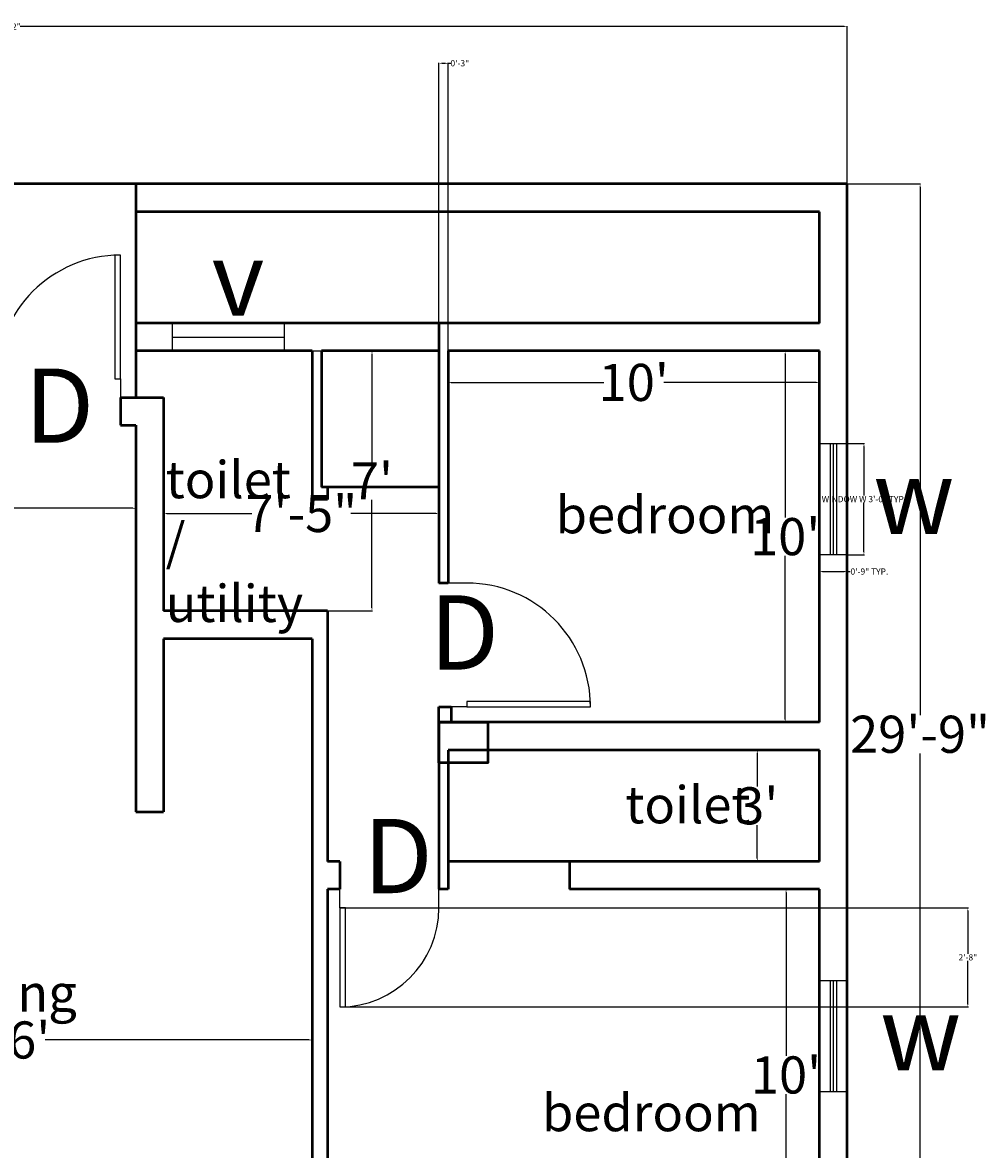
# Model space of a CAD drawing. Units: inches. Extents: x 409 to 7572, y 7 to 725.
# Tile 6 of 38: x 860 to 1171, y 360 to 725. Entities that reach past the tile are written whole.
import ezdxf

# ---------------------------------------------------------------- set-up
doc = ezdxf.new("R2010")
doc.units = ezdxf.units.IN
doc.header["$MEASUREMENT"] = 0
for name, color, linetype, lineweight in [('A-ANNO-DIMS', 2, 'Continuous', 18), ('A-ANNO-SYMB', 3, 'Continuous', 25), ('A-AREA-IDEN', 7, 'Continuous', 25), ('A-DOOR', 3, 'Continuous', 25), ('A-GLAZ', 4, 'Continuous', 25), ('A-WALL', 7, 'Continuous', 50)]:
    doc.layers.add(name, color=color, linetype=linetype, lineweight=lineweight)
doc.styles.get("Standard").update_dxf_attribs({"font": 'arial.ttf'})
doc.dimstyles.get("Standard").update_dxf_attribs({"dimtxt": 2, "dimasz": 1, "dimexe": 0.18, "dimexo": 0.0625, "dimgap": 0.09, "dimtad": 0, "dimtih": 1, "dimtoh": 1, "dimdec": 0, "dimzin": 0, "dimdsep": 46, "dimlunit": 3, "dimtxsty": 'Standard', "dimcen": 0.09, "dimadec": 0, "dimazin": 0, "dimtfac": 1, "dimtdec": 0, "dimtofl": 0, "dimtmove": 0, "dimatfit": 3, "dimfxl": 1, "dimtolj": 1, "dimtzin": 0, "dimarcsym": 0})

# ---------------------------------------------------------------- blocks, each defined once
blk = doc.blocks.new('*U2')
for p, q in [((0, 0), (0, -6)), ((-40, 0), (-40, -6))]:
    blk.add_line(p, q)
blk.add_lwpolyline([(0, 0), (0, 40), (-1.75, 40), (-1.75, 0)], close=True)
blk.add_arc((0, 0), 40, 90, 180)
blk = doc.blocks.new('*U6')
for p, q in [((0, 0), (0, -6)), ((-40, 0), (-40, -6))]:
    blk.add_line(p, q)
blk.add_lwpolyline([(0, 0), (0, 40), (-1.75, 40), (-1.75, 0)], close=True)
blk.add_arc((0, 0), 40, 90, 180)
blk = doc.blocks.new('*U7')
for p, q in [((0, 0), (0, 6)), ((32, 0), (32, 6))]:
    blk.add_line(p, q)
blk.add_lwpolyline([(0, 0), (0, -32), (1.75, -32), (1.75, 0)], close=True)
blk.add_arc((0, 0), 32, 270, 0)
blk = doc.blocks.new('*D11')
at = {"layer": 'A-ANNO-DIMS', "color": 0, "lineweight": -2, "transparency": 16777216}
for p, q in [((997.16, 618.47), (997.16, 608.19)), ((1117.16, 618.47), (1117.16, 608.19)), ((998.16, 608.37), (1047.45, 608.37)), ((1116.16, 608.37), (1066.86, 608.37))]:
    blk.add_line(p, q, dxfattribs=at)
at = {"layer": 'A-ANNO-DIMS', "color": 0, "transparency": 16777216}
for points in [[(998.16, 608.54), (998.16, 608.2), (997.16, 608.37)], [(1116.16, 608.54), (1116.16, 608.2), (1117.16, 608.37)]]:
    blk.add_solid(points, dxfattribs=at)
at = {"layer": 'DEFPOINTS', "color": 0, "transparency": 16777216}
for p in [(997.16, 618.53), (1117.16, 618.53), (997.16, 608.37)]:
    blk.add_point(p, dxfattribs=at)
at = {"layer": 'A-ANNO-DIMS', "color": 0, "transparency": 16777216, "insert": (1057.16, 608.37), "char_height": 2, "attachment_point": 5}
blk.add_mtext("\\A1;{\\H6x;10'}", dxfattribs=at)
blk = doc.blocks.new('*D12')
at = {"layer": 'A-ANNO-DIMS', "color": 0, "lineweight": -2, "transparency": 16777216}
for p, q in [((1117.09, 618.53), (1105.93, 618.53)), ((1106.11, 617.53), (1106.11, 564.75)), ((1106.11, 499.53), (1106.11, 552.31)), ((1117.09, 498.53), (1105.93, 498.53))]:
    blk.add_line(p, q, dxfattribs=at)
at = {"layer": 'A-ANNO-DIMS', "color": 0, "transparency": 16777216}
for points in [[(1105.94, 617.53), (1106.27, 617.53), (1106.11, 618.53)], [(1105.94, 499.53), (1106.27, 499.53), (1106.11, 498.53)]]:
    blk.add_solid(points, dxfattribs=at)
at = {"layer": 'DEFPOINTS', "color": 0, "transparency": 16777216}
for p in [(1106.11, 618.53), (1117.16, 618.53), (1117.16, 498.53)]:
    blk.add_point(p, dxfattribs=at)
at = {"layer": 'A-ANNO-DIMS', "color": 0, "transparency": 16777216, "insert": (1106.11, 558.53), "char_height": 2, "attachment_point": 5}
blk.add_mtext("\\A1;{\\H6x;10'}", dxfattribs=at)
blk = doc.blocks.new('*D13')
at = {"layer": 'A-ANNO-DIMS', "color": 0, "lineweight": -2, "transparency": 16777216}
for p, q in [((1117.09, 444.53), (1106.21, 444.53)), ((1106.39, 443.53), (1106.39, 390.75)), ((1106.39, 325.53), (1106.39, 378.31)), ((1117.09, 324.53), (1106.21, 324.53))]:
    blk.add_line(p, q, dxfattribs=at)
at = {"layer": 'A-ANNO-DIMS', "color": 0, "transparency": 16777216}
for points in [[(1106.22, 443.53), (1106.56, 443.53), (1106.39, 444.53)], [(1106.22, 325.53), (1106.56, 325.53), (1106.39, 324.53)]]:
    blk.add_solid(points, dxfattribs=at)
at = {"layer": 'DEFPOINTS', "color": 0, "transparency": 16777216}
for p in [(1106.39, 444.53), (1117.16, 444.53), (1117.16, 324.53)]:
    blk.add_point(p, dxfattribs=at)
at = {"layer": 'A-ANNO-DIMS', "color": 0, "transparency": 16777216, "insert": (1106.39, 384.53), "char_height": 2, "attachment_point": 5}
blk.add_mtext("\\A1;{\\H6x;10'}", dxfattribs=at)
blk = doc.blocks.new('*D22')
at = {"layer": 'A-ANNO-DIMS', "color": 0, "lineweight": -2, "transparency": 16777216}
for p, q in [((761.16, 563.4), (761.16, 567.87)), ((762.16, 567.69), (808.52, 567.69)), ((895.16, 567.69), (848.79, 567.69)), ((896.16, 563.4), (896.16, 567.87))]:
    blk.add_line(p, q, dxfattribs=at)
at = {"layer": 'A-ANNO-DIMS', "color": 0, "transparency": 16777216}
for points in [[(762.16, 567.86), (762.16, 567.52), (761.16, 567.69)], [(895.16, 567.86), (895.16, 567.52), (896.16, 567.69)]]:
    blk.add_solid(points, dxfattribs=at)
at = {"layer": 'DEFPOINTS', "color": 0, "transparency": 16777216}
for p in [(896.16, 567.69), (761.16, 563.33), (896.16, 563.33)]:
    blk.add_point(p, dxfattribs=at)
at = {"layer": 'A-ANNO-DIMS', "color": 0, "transparency": 16777216, "insert": (828.66, 567.69), "char_height": 2, "attachment_point": 5}
blk.add_mtext('\\A1;{\\H6x;11\'-3"}', dxfattribs=at)
blk = doc.blocks.new('*D23')
at = {"layer": 'A-ANNO-DIMS', "color": 0, "lineweight": -2, "transparency": 16777216}
for p, q in [((761.16, 403.47), (761.16, 395.65)), ((953.16, 403.47), (953.16, 395.65)), ((762.16, 395.83), (847.45, 395.83)), ((952.16, 395.83), (866.86, 395.83))]:
    blk.add_line(p, q, dxfattribs=at)
at = {"layer": 'A-ANNO-DIMS', "color": 0, "transparency": 16777216}
for points in [[(762.16, 396), (762.16, 395.66), (761.16, 395.83)], [(952.16, 396), (952.16, 395.66), (953.16, 395.83)]]:
    blk.add_solid(points, dxfattribs=at)
at = {"layer": 'DEFPOINTS', "color": 0, "transparency": 16777216}
for p in [(761.16, 403.53), (953.16, 403.53), (953.16, 395.83)]:
    blk.add_point(p, dxfattribs=at)
at = {"layer": 'A-ANNO-DIMS', "color": 0, "transparency": 16777216, "insert": (857.16, 395.83), "char_height": 2, "attachment_point": 5}
blk.add_mtext("\\A1;{\\H6x;16'}", dxfattribs=at)
blk = doc.blocks.new('*D25')
at = {"layer": 'A-ANNO-DIMS', "color": 0, "lineweight": -2, "transparency": 16777216}
for p, q in [((905.16, 568.97), (905.16, 565.83)), ((994.16, 568.97), (994.16, 565.83)), ((906.16, 566.01), (933.67, 566.01)), ((993.16, 566.01), (965.65, 566.01))]:
    blk.add_line(p, q, dxfattribs=at)
at = {"layer": 'A-ANNO-DIMS', "color": 0, "transparency": 16777216}
for points in [[(906.16, 566.17), (906.16, 565.84), (905.16, 566.01)], [(993.16, 566.17), (993.16, 565.84), (994.16, 566.01)]]:
    blk.add_solid(points, dxfattribs=at)
at = {"layer": 'DEFPOINTS', "color": 0, "transparency": 16777216}
for p in [(905.16, 569.03), (994.16, 569.03), (994.16, 566.01)]:
    blk.add_point(p, dxfattribs=at)
at = {"layer": 'A-ANNO-DIMS', "color": 0, "transparency": 16777216, "insert": (949.66, 566.01), "char_height": 2, "attachment_point": 5}
blk.add_mtext('\\A1;{\\H6x;7\'-5"}', dxfattribs=at)
blk = doc.blocks.new('*D26')
at = {"layer": 'A-ANNO-DIMS', "color": 0, "lineweight": -2, "transparency": 16777216}
for p, q in [((924.72, 618.53), (972.69, 618.53)), ((972.51, 617.53), (972.51, 582.62)), ((972.51, 535.53), (972.51, 570.44)), ((924.72, 534.53), (972.69, 534.53))]:
    blk.add_line(p, q, dxfattribs=at)
at = {"layer": 'A-ANNO-DIMS', "color": 0, "transparency": 16777216}
for points in [[(972.35, 617.53), (972.68, 617.53), (972.51, 618.53)], [(972.35, 535.53), (972.68, 535.53), (972.51, 534.53)]]:
    blk.add_solid(points, dxfattribs=at)
at = {"layer": 'DEFPOINTS', "color": 0, "transparency": 16777216}
for p in [(924.66, 618.53), (924.66, 534.53), (972.51, 534.53)]:
    blk.add_point(p, dxfattribs=at)
at = {"layer": 'A-ANNO-DIMS', "color": 0, "transparency": 16777216, "insert": (972.51, 576.53), "char_height": 2, "attachment_point": 5}
blk.add_mtext("\\A1;{\\H6x;7'}", dxfattribs=at)
blk = doc.blocks.new('*D28')
at = {"layer": 'A-ANNO-DIMS', "color": 0, "lineweight": -2, "transparency": 16777216}
for p, q in [((1117.09, 489.53), (1096.9, 489.53)), ((1097.08, 488.53), (1097.08, 477.75)), ((1097.08, 454.53), (1097.08, 465.31)), ((1117.09, 453.53), (1096.9, 453.53))]:
    blk.add_line(p, q, dxfattribs=at)
at = {"layer": 'A-ANNO-DIMS', "color": 0, "transparency": 16777216}
for points in [[(1096.92, 488.53), (1097.25, 488.53), (1097.08, 489.53)], [(1096.92, 454.53), (1097.25, 454.53), (1097.08, 453.53)]]:
    blk.add_solid(points, dxfattribs=at)
at = {"layer": 'DEFPOINTS', "color": 0, "transparency": 16777216}
for p in [(1117.16, 489.53), (1097.08, 453.53), (1117.16, 453.53)]:
    blk.add_point(p, dxfattribs=at)
at = {"layer": 'A-ANNO-DIMS', "color": 0, "transparency": 16777216, "insert": (1097.08, 471.53), "char_height": 2, "attachment_point": 5}
blk.add_mtext("\\A1;{\\H6x;3'}", dxfattribs=at)
blk = doc.blocks.new('*D30')
at = {"layer": 'A-ANNO-DIMS', "color": 0, "lineweight": -2, "transparency": 16777216}
for p, q in [((584.16, 672.59), (584.16, 723.56)), ((585.16, 723.38), (851.59, 723.38)), ((1125.16, 723.38), (858.72, 723.38)), ((1126.16, 672.59), (1126.16, 723.56))]:
    blk.add_line(p, q, dxfattribs=at)
at = {"layer": 'A-ANNO-DIMS', "color": 0, "transparency": 16777216}
for points in [[(585.16, 723.55), (585.16, 723.22), (584.16, 723.38)], [(1125.16, 723.55), (1125.16, 723.22), (1126.16, 723.38)]]:
    blk.add_solid(points, dxfattribs=at)
at = {"layer": 'DEFPOINTS', "color": 0, "transparency": 16777216}
for p in [(584.16, 723.38), (584.16, 672.53), (1126.16, 672.53)]:
    blk.add_point(p, dxfattribs=at)
at = {"layer": 'A-ANNO-DIMS', "color": 0, "transparency": 16777216, "insert": (855.16, 723.38), "char_height": 2, "attachment_point": 5}
blk.add_mtext('\\A1;45\'-2"', dxfattribs=at)
blk = doc.blocks.new('*D35')
at = {"layer": 'A-ANNO-DIMS', "color": 0, "lineweight": -2, "transparency": 16777216}
for p, q in [((1126.22, 672.53), (1149.9, 672.53)), ((1149.72, 671.53), (1149.72, 500.86)), ((1149.72, 316.53), (1149.72, 488.43)), ((1126.22, 315.53), (1149.9, 315.53))]:
    blk.add_line(p, q, dxfattribs=at)
at = {"layer": 'A-ANNO-DIMS', "color": 0, "transparency": 16777216}
for points in [[(1149.56, 671.53), (1149.89, 671.53), (1149.72, 672.53)], [(1149.56, 316.53), (1149.89, 316.53), (1149.72, 315.53)]]:
    blk.add_solid(points, dxfattribs=at)
at = {"layer": 'DEFPOINTS', "color": 0, "transparency": 16777216}
for p in [(1126.16, 672.53), (1149.72, 672.53), (1126.16, 315.53)]:
    blk.add_point(p, dxfattribs=at)
at = {"layer": 'A-ANNO-DIMS', "color": 0, "transparency": 16777216, "insert": (1149.72, 494.65), "char_height": 2, "attachment_point": 5}
blk.add_mtext('\\A1;{\\H6x;29\'-9"}', dxfattribs=at)
blk = doc.blocks.new('WIN-36')
for p, q in [((1699.82, 514.65), (1699.82, 478.65)), ((1700.82, 514.65), (1700.82, 478.65)), ((1701.82, 514.65), (1701.82, 478.65))]:
    blk.add_line(p, q)
blk.add_lwpolyline([(1705.32, 514.65), (1705.32, 478.65), (1696.32, 478.65), (1696.32, 514.65)], close=True)
blk = doc.blocks.new('VENT-36')
blk.add_line((5633.28, 355.73), (5633.28, 391.73))
blk.add_lwpolyline([(5628.78, 355.73), (5628.78, 391.73), (5637.78, 391.73), (5637.78, 355.73)], close=True)
blk = doc.blocks.new('*D167')
at = {"layer": 'A-ANNO-DIMS', "color": 0, "lineweight": -2, "transparency": 16777216}
for p, q in [((1126.22, 588.64), (1131.74, 588.64)), ((1131.56, 587.64), (1131.56, 571.77)), ((1131.56, 553.64), (1131.56, 569.51)), ((1126.22, 552.64), (1131.74, 552.64))]:
    blk.add_line(p, q, dxfattribs=at)
at = {"layer": 'A-ANNO-DIMS', "color": 0, "transparency": 16777216}
for points in [[(1131.39, 587.64), (1131.72, 587.64), (1131.56, 588.64)], [(1131.39, 553.64), (1131.72, 553.64), (1131.56, 552.64)]]:
    blk.add_solid(points, dxfattribs=at)
at = {"layer": 'DEFPOINTS', "color": 0, "transparency": 16777216}
for p in [(1126.16, 588.64), (1131.56, 588.64), (1126.16, 552.64)]:
    blk.add_point(p, dxfattribs=at)
at = {"layer": 'A-ANNO-DIMS', "color": 0, "transparency": 16777216, "insert": (1131.56, 570.64), "char_height": 2, "attachment_point": 5}
blk.add_mtext('\\A1;WINDOW W 3\'-0" TYP.', dxfattribs=at)
blk = doc.blocks.new('*D168')
at = {"layer": 'A-ANNO-DIMS', "color": 0, "lineweight": -2, "transparency": 16777216}
for p, q in [((1117.16, 552.58), (1117.16, 547.06)), ((1126.16, 552.58), (1126.16, 547.06)), ((1118.16, 547.24), (1125.16, 547.24)), ((1126.16, 547.24), (1127.16, 547.24))]:
    blk.add_line(p, q, dxfattribs=at)
at = {"layer": 'A-ANNO-DIMS', "color": 0, "transparency": 16777216}
for points in [[(1118.16, 547.41), (1118.16, 547.07), (1117.16, 547.24)], [(1125.16, 547.41), (1125.16, 547.07), (1126.16, 547.24)]]:
    blk.add_solid(points, dxfattribs=at)
at = {"layer": 'DEFPOINTS', "color": 0, "transparency": 16777216}
for p in [(1117.16, 552.64), (1126.16, 552.64), (1126.16, 547.24)]:
    blk.add_point(p, dxfattribs=at)
at = {"layer": 'A-ANNO-DIMS', "color": 0, "transparency": 16777216, "insert": (1133.34, 547.24), "char_height": 2, "attachment_point": 5}
blk.add_mtext('\\A1;0\'-9" TYP.', dxfattribs=at)
blk = doc.blocks.new('*D175')
at = {"layer": 'A-ANNO-DIMS', "color": 0, "lineweight": -2, "transparency": 16777216}
for p, q in [((994.16, 627.59), (994.16, 711.71)), ((995.16, 711.53), (996.16, 711.53)), ((997.16, 618.59), (997.16, 711.71)), ((997.16, 711.53), (998.16, 711.53))]:
    blk.add_line(p, q, dxfattribs=at)
at = {"layer": 'A-ANNO-DIMS', "color": 0, "transparency": 16777216}
for points in [[(995.16, 711.7), (995.16, 711.36), (994.16, 711.53)], [(996.16, 711.7), (996.16, 711.36), (997.16, 711.53)]]:
    blk.add_solid(points, dxfattribs=at)
at = {"layer": 'DEFPOINTS', "color": 0, "transparency": 16777216}
for p in [(997.16, 711.53), (994.16, 627.53), (997.16, 618.53)]:
    blk.add_point(p, dxfattribs=at)
at = {"layer": 'A-ANNO-DIMS', "color": 0, "transparency": 16777216, "insert": (1000.9, 711.53), "char_height": 2, "attachment_point": 5}
blk.add_mtext('\\A1;0\'-3"', dxfattribs=at)
blk = doc.blocks.new('*D176')
at = {"layer": 'A-ANNO-DIMS', "color": 0, "lineweight": -2, "transparency": 16777216}
for p, q in [((962.22, 438.53), (1165.34, 438.53)), ((1165.16, 437.53), (1165.16, 423.64)), ((1165.16, 407.53), (1165.16, 421.42)), ((962.22, 406.53), (1165.34, 406.53))]:
    blk.add_line(p, q, dxfattribs=at)
at = {"layer": 'A-ANNO-DIMS', "color": 0, "transparency": 16777216}
for points in [[(1164.99, 437.53), (1165.32, 437.53), (1165.16, 438.53)], [(1164.99, 407.53), (1165.32, 407.53), (1165.16, 406.53)]]:
    blk.add_solid(points, dxfattribs=at)
at = {"layer": 'DEFPOINTS', "color": 0, "transparency": 16777216}
for p in [(962.16, 438.53), (962.16, 406.53), (1165.16, 406.53)]:
    blk.add_point(p, dxfattribs=at)
at = {"layer": 'A-ANNO-DIMS', "color": 0, "transparency": 16777216, "insert": (1165.16, 422.53), "char_height": 2, "attachment_point": 5}
blk.add_mtext('\\A1;2\'-8"', dxfattribs=at)

msp = doc.modelspace()

# ---------------------------------------------------------------- linework, layer by layer
at = {"layer": 'A-WALL'}
for p, q in [((1126.16, 672.53), (584.16, 672.53)), ((896.16, 672.53), (896.16, 603.53)), ((1126.16, 315.53), (1126.16, 672.53)), ((1117.16, 663.53), (896.16, 663.53)), ((1117.16, 627.53), (1117.16, 663.53)), ((1117.16, 627.53), (896.16, 627.53)), ((994.16, 627.53), (994.16, 543.53)), ((953.16, 618.53), (896.16, 618.53)), ((953.16, 618.53), (953.16, 570.53)), ((956.16, 618.53), (956.16, 574.53)), ((994.16, 618.53), (956.16, 618.53)), ((1117.16, 618.53), (997.16, 618.53)), ((997.16, 618.53), (997.16, 543.53)), ((1117.16, 498.53), (1117.16, 618.53)), ((891.16, 603.53), (905.16, 603.53)), ((891.16, 603.53), (891.16, 594.53)), ((905.16, 603.53), (905.16, 534.53)), ((891.16, 594.53), (896.16, 594.53)), ((994.16, 574.53), (956.16, 574.53)), ((958.16, 574.53), (958.16, 570.53)), ((958.16, 570.53), (953.16, 570.53)), ((997.16, 543.53), (994.16, 543.53)), ((958.16, 534.53), (905.16, 534.53)), ((958.16, 534.53), (958.16, 453.53)), ((953.16, 525.53), (905.16, 525.53)), ((905.16, 525.53), (905.16, 469.53)), ((953.16, 525.53), (953.16, 337.53)), ((994.16, 498.53), (994.16, 503.53)), ((994.16, 503.53), (998.16, 503.53)), ((998.16, 503.53), (998.16, 498.53)), ((1117.16, 498.53), (994.16, 498.53)), ((994.16, 498.53), (994.16, 444.53)), ((953.16, 489.53), (953.16, 337.53)), ((1117.16, 489.53), (997.16, 489.53)), ((997.16, 489.53), (997.16, 444.53)), ((1117.16, 453.53), (1117.16, 489.53)), ((896.16, 469.53), (905.16, 469.53)), ((962.16, 453.53), (958.16, 453.53)), ((962.16, 453.53), (962.16, 444.53)), ((1117.16, 453.53), (997.16, 453.53)), ((1036.35, 453.53), (1036.35, 444.53)), ((962.16, 444.53), (958.16, 444.53)), ((958.16, 444.53), (958.16, 324.53)), ((997.16, 444.53), (994.16, 444.53)), ((997.16, 444.53), (994.16, 444.53)), ((1117.16, 444.53), (1036.35, 444.53)), ((1117.16, 324.53), (1117.16, 444.53))]:
    msp.add_line(p, q, dxfattribs=at)
msp.add_lwpolyline([(896.16, 594.53), (896.16, 525.53), (896.16, 469.53)], dxfattribs=at)
msp.add_lwpolyline([(994.16, 498.53), (1010.02, 498.53), (1010.02, 485.36), (994.16, 485.36)], close=True, dxfattribs=at)

# ---------------------------------------------------------------- block references
at = {"layer": 'A-DOOR'}
for name, p in [('*U2', (891.16, 609.53)), ('*U7', (962.16, 438.53))]:
    msp.add_blockref(name, p, dxfattribs=at)
at = {"layer": 'A-DOOR', "rotation": 270}
msp.add_blockref('*U6', (1003.16, 503.53), dxfattribs=at)
at = {"layer": 'A-GLAZ', "rotation": 269.9999999999993}
msp.add_blockref('VENT-36', (552.34, 6256.31), dxfattribs=at)
at = {"layer": 'A-GLAZ'}
for p in [(-579.16, 73.99), (-579.16, -99.57)]:
    msp.add_blockref('WIN-36', p, dxfattribs=at)

# ---------------------------------------------------------------- texts
at = {"layer": 'A-ANNO-SYMB', "char_height": 24, "attachment_point": 1}
for s, width, insert in [('v', 18.2582, (920.66, 653.91)), ('D', 19.1972, (860.18, 612.87)), ('w', 18.2582, (1134.56, 583.33)), ('D', 19.1972, (991.08, 539.54)), ('D', 19.1972, (969.66, 467.28)), ('w', 18.2582, (1136.76, 410.07))]:
    msp.add_mtext_dynamic_manual_height_columns(s, width=width, gutter_width=1, heights=[0], dxfattribs=dict(at, insert=insert))
at = {"layer": 'A-AREA-IDEN', "char_height": 12, "attachment_point": 1}
for s, width, insert in [('toilet / utility', 49.2946, (905.81, 582.94)), ('bedroom', 40.9017, (1031.91, 571.6)), ('toilet', 49.2946, (1054.41, 477.86)), ('Dining ', 67.5069, (827.59, 417.03)), ('bedroom', 40.9017, (1027.49, 378.34))]:
    msp.add_mtext_dynamic_manual_height_columns(s, width=width, gutter_width=1, heights=[0], dxfattribs=dict(at, insert=insert))

# ---------------------------------------------------------------- dimensions: what is measured, and where the dimension line sits
at = {"layer": 'A-ANNO-DIMS'}
for base, p1, p2, override, picture, middle in [((584.16, 723.38), (1126.16, 672.53), (584.16, 672.53), {"dimclrd": 0, "dimclre": 0, "dimclrt": 0}, '*D30', (855.16, 723.38)), ((997.16, 711.53), (994.16, 627.53), (997.16, 618.53), {"dimdec": 1, "dimlfac": 1, "dimrnd": 0, "dimzin": 1, "dimdsep": 46, "dimlunit": 4, "dimfrac": 2}, '*D175', (1000.9, 711.53))]:
    dim = msp.add_linear_dim(base=base, p1=p1, p2=p2, dimstyle='Standard', override=override, dxfattribs=at)
    dim.commit()
    dim.dimension.update_dxf_attribs({"geometry": picture, "text_midpoint": middle})
dim = msp.add_linear_dim(base=(1149.72, 672.53), p1=(1126.16, 315.53), p2=(1126.16, 672.53), angle=90, text='{\\H6x;<>}', dimstyle='Standard', override={"dimclrd": 0, "dimclre": 0, "dimclrt": 0}, dxfattribs=at)
dim.commit()
dim.dimension.update_dxf_attribs({"geometry": '*D35', "text_midpoint": (1149.72, 494.65), "dimtype": 160})
for base, p1, p2, text, override, picture, middle in [((972.51, 534.53), (924.66, 618.53), (924.66, 534.53), '{\\H6x;<>}', {"dimclrd": 0, "dimclre": 0, "dimclrt": 0}, '*D26', (972.51, 576.53)), ((1106.11, 618.53), (1117.16, 498.53), (1117.16, 618.53), '{\\H6x;<>}', {"dimclrd": 0, "dimclre": 0, "dimclrt": 0}, '*D12', (1106.11, 558.53)), ((1131.56, 588.64), (1126.16, 552.64), (1126.16, 588.64), 'WINDOW W <> TYP.', {"dimdec": 1, "dimrnd": 0, "dimzin": 1, "dimlunit": 4, "dimfrac": 2}, '*D167', (1131.56, 570.64)), ((1097.08, 453.53), (1117.16, 489.53), (1117.16, 453.53), '{\\H6x;<>}', {"dimclrd": 0, "dimclre": 0, "dimclrt": 0}, '*D28', (1097.08, 471.53)), ((1106.39, 444.53), (1117.16, 324.53), (1117.16, 444.53), '{\\H6x;<>}', {"dimclrd": 0, "dimclre": 0, "dimclrt": 0}, '*D13', (1106.39, 384.53))]:
    dim = msp.add_linear_dim(base=base, p1=p1, p2=p2, angle=90, text=text, dimstyle='Standard', override=override, dxfattribs=at)
    dim.commit()
    dim.dimension.update_dxf_attribs({"geometry": picture, "text_midpoint": middle})
for base, p1, p2, text, override, picture, middle in [((997.16, 608.37), (1117.16, 618.53), (997.16, 618.53), '{\\H6x;<>}', {"dimclrd": 0, "dimclre": 0, "dimclrt": 0}, '*D11', (1057.16, 608.37)), ((896.16, 567.69), (761.16, 563.33), (896.16, 563.33), '{\\H6x;<>}', {"dimclrd": 0, "dimclre": 0, "dimclrt": 0}, '*D22', (828.66, 567.69)), ((994.16, 566.01), (905.16, 569.03), (994.16, 569.03), '{\\H6x;<>}', {"dimclrd": 0, "dimclre": 0, "dimclrt": 0}, '*D25', (949.66, 566.01)), ((1126.16, 547.24), (1117.16, 552.64), (1126.16, 552.64), '<> TYP.', {"dimdec": 1, "dimrnd": 0, "dimzin": 1, "dimlunit": 4, "dimfrac": 2}, '*D168', (1133.34, 547.24))]:
    dim = msp.add_linear_dim(base=base, p1=p1, p2=p2, text=text, dimstyle='Standard', override=override, dxfattribs=at)
    dim.commit()
    dim.dimension.update_dxf_attribs({"geometry": picture, "text_midpoint": middle})
dim = msp.add_linear_dim(base=(1165.16, 406.53), p1=(962.16, 438.53), p2=(962.16, 406.53), angle=90, dimstyle='Standard', override={"dimdec": 1, "dimlfac": 1, "dimrnd": 0, "dimzin": 1, "dimdsep": 46, "dimlunit": 4, "dimfrac": 2}, dxfattribs=at)
dim.commit()
dim.dimension.update_dxf_attribs({"geometry": '*D176', "text_midpoint": (1165.16, 422.53)})
dim = msp.add_linear_dim(base=(953.16, 395.83), p1=(761.16, 403.53), p2=(953.16, 403.53), text='{\\H6x;<>}', dimstyle='Standard', override={"dimclrd": 0, "dimclre": 0, "dimclrt": 0}, dxfattribs=at)
dim.commit()
dim.dimension.update_dxf_attribs({"geometry": '*D23', "text_midpoint": (857.16, 395.83), "dimtype": 160})

doc.saveas('drawing.dxf')
